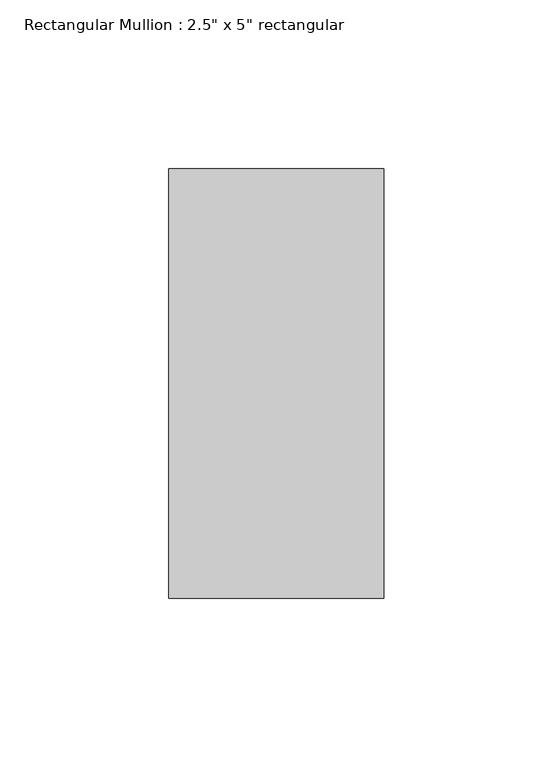
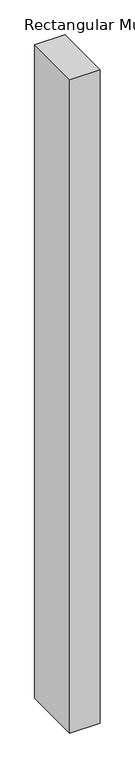
"""IFC4 building model written with IfcOpenShell, lengths in millimetres: member geometry."""

from ifc_helpers import new_model, si_unit, frame, origin, place, context, project, spatial, polyline, outline, extrude, source, transform, mapped, element, save


def member_a4862887(model_context):
    return source(origin(), model_context, "Body", "SweptSolid", [
        extrude(outline(polyline([(31.75, 63.5), (31.75, -63.5), (-31.75, -63.5), (-31.75, 63.5), (31.75, 63.5)])), frame((0.0, 0.0, -1447.0507887), z_axis=(0.0, 0.0, 1.0), x_axis=(1.0, 0.0, 0.0)), (0.0, 0.0, 1.0), 1447.0507887),
    ])


if __name__ == "__main__":
    model = new_model("IFC4")
    model_context = context("Model", 3, world=origin())
    ifc_project = project(units=[si_unit("LENGTHUNIT", "METRE", prefix="MILLI")], contexts=[model_context])
    site = spatial("IfcSite", under=ifc_project)
    building = spatial("IfcBuilding", under=site)
    placement = place(None, origin())
    member_shape = member_a4862887(model_context)
    element("IfcMember", 1, ObjectType="Rectangular Mullion : 2.5\" x 5\" rectangular", at=placement, inside=building, context=model_context, shape_type="MappedRepresentation", body=[
        mapped(member_shape, transform((0.0, 0.0, 0.0), x_axis=(1.0, 0.0, 0.0), y_axis=(0.0, 1.0, 0.0), z_axis=(0.0, 0.0, 1.0))),
    ])
    save(model, "model.ifc")

# Revit data of these elements
# Type "Rectangular Mullion : 2.5\" x 5\" rectangular"
#   built-in parameter 1007304 = 0.416667 (stored number, unit not read)
#   built-in parameter 1007301 = 0.104167 (stored number, unit not read)
#   built-in parameter 1007300 = 0.104167 (stored number, unit not read)
# Element 1 (IfcMember, "Rectangular Mullion : 2.5\" x 5\" rectangular")
#   Materials on its faces: "Aluminum"
# Materials
#   "Aluminum": class "Metal", colour RGB 247 247 247, transparency 0, Description = "Aluminum 6061", Cost = 0
